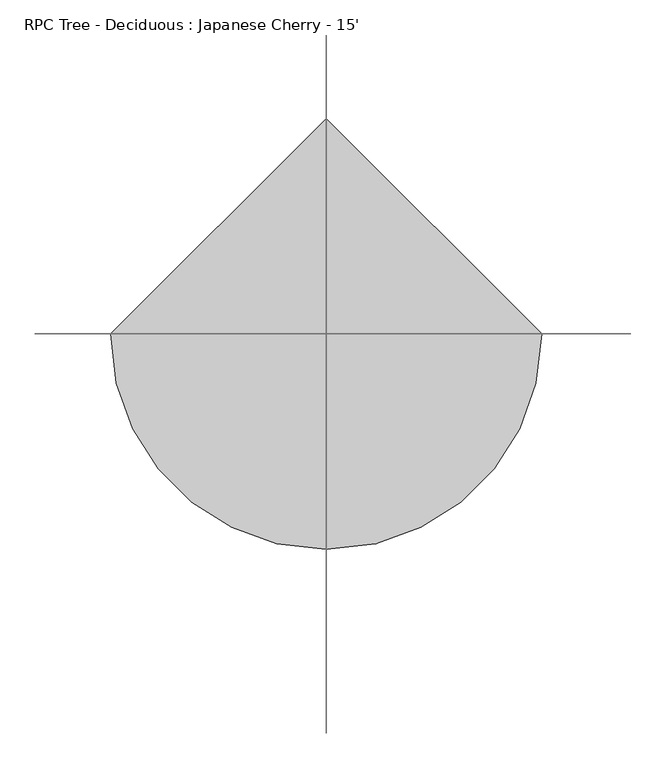
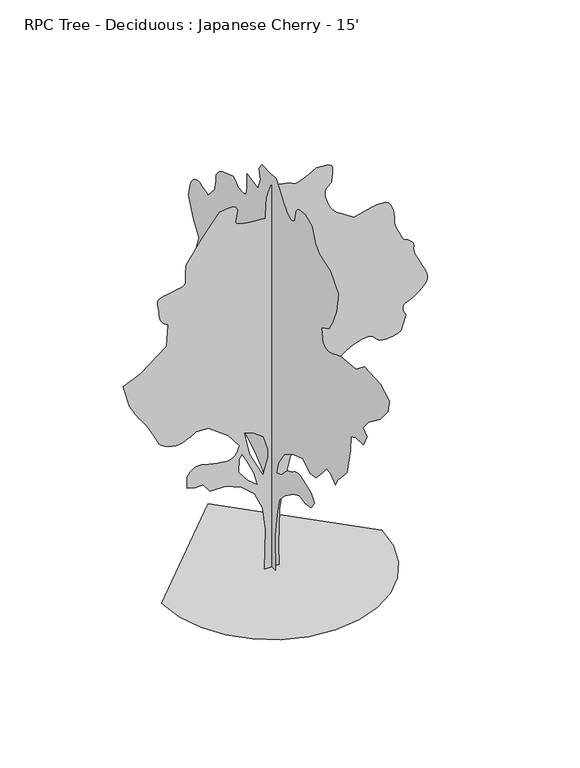
"""IFC4 building model written with IfcOpenShell, lengths in millimetres: geographic element geometry, RPC Tree - Deciduous : Japanese Cherry - 15'."""

from ifc_helpers import new_model, si_unit, origin, place, context, project, spatial, triangles, source, transform, mapped, element, save


def rpc_tree_deciduous_japanese_cherry_15_4daa029f(model_context):
    return source(origin(), model_context, "Body", "Tessellation", [
        triangles([(-0.0056056, 151.5314393, 0.0119075), (-0.0056056, -146.4956366, 0.0119075), (-0.0056056, -119.4024502, 799.2624058), (-0.0056056, -200.6820093, 1327.5829193), (-0.0056056, -295.5089247, 1733.9832584), (-0.0056056, -512.2574678, 1964.2750156), (-0.0056056, -837.3726522, 2194.5718597), (-0.0056056, -1054.1211954, 2289.3952869), (-0.0056056, -1270.8696659, 2248.7551804), (-0.0056056, -1501.1615685, 2289.3952869), (-0.0056056, -1623.0815975, 2465.5038689), (-0.0056056, -1501.1615685, 2628.0640045), (-0.0056056, -1067.669569, 2777.0755486), (-0.0056056, -1029.9911276, 2774.0379433), (-0.0056056, -992.6683331, 2770.1669586), (-0.0056056, -956.0567596, 2764.6347382), (-0.0056056, -920.5119816, 2756.618367), (-0.0056056, -886.3895731, 2745.2850471), (-0.0056056, -854.0400942, 2729.8011086), (-0.0056056, -823.8293655, 2709.343927), (-0.0056056, -793.6134773, 2687.3069), (-0.0056056, -761.2690853, 2667.3982315), (-0.0056056, -727.1466768, 2649.2728844), (-0.0056056, -691.6018988, 2632.5648926), (-0.0056056, -654.9903254, 2616.9286377), (-0.0056056, -617.6675308, 2601.9984444), (-0.0056056, -579.9891621, 2587.4237526), (-0.0056056, -376.7884838, 2370.6753548), (-0.0056056, -173.5888229, 2289.3952869), (-0.0056056, -254.8688908, 2573.8754517), (-0.0056056, -485.161738, 2912.5440239), (-0.0056056, -810.2809919, 3115.7444115), (-0.0056056, -1189.5895981, 3237.6642952), (-0.0056056, -1460.5214619, 3061.5558586), (-0.0056056, -1677.270005, 3088.6527512), (-0.0056056, -1907.5619076, 3332.4878677), (-0.0056056, -2083.6703442, 3549.2362656), (-0.0056056, -2246.2253929, 3535.6879646), (-0.0056056, -2422.3338295, 3373.1327705), (-0.0056056, -2530.705703, 3562.7845665), (-0.0056056, -2652.6255867, 3698.2481003), (-0.0056056, -2869.3742752, 3928.544799), (-0.0056056, -3004.8375183, 4538.1453804), (-0.0056056, -3018.3861099, 4863.2656517), (-0.0056056, -3208.0428474, 4944.5406326), (-0.0056056, -3506.0665169, 4971.6372345), (-0.0056056, -3627.9864006, 5229.0005951), (-0.0056056, -3478.9748566, 5350.9204788), (-0.0056056, -3682.1749535, 5594.7608276), (-0.0056056, -4142.7584679, 5947.0085129), (-0.0056056, -4440.7870789, 6299.2050385), (-0.0056056, -4494.9703995, 6583.6853485), (-0.0056056, -4156.3070595, 6773.3220291), (-0.0056056, -3533.1581772, 6800.4488617), (-0.0056056, -3221.5862068, 6556.6090942), (-0.0056056, -2625.5339264, 6488.8417191), (-0.0056056, -2544.569101, 6457.0913315), (-0.0056056, -2465.5038689, 6426.4083206), (-0.0056056, -2390.2231441, 6397.8589005), (-0.0056056, -2320.6372753, 6372.509285), (-0.0056056, -2258.6307404, 6351.4274323), (-0.0056056, -2206.1035686, 6335.6795563), (-0.0056056, -2164.9453251, 6326.2812927), (-0.0056056, -2128.100045, 6325.7731842), (-0.0056056, -2089.1160873, 6333.8000198), (-0.0056056, -2050.8485104, 6347.2619888), (-0.0056056, -2016.1317341, 6363.1116028), (-0.0056056, -1987.8157299, 6378.2496323), (-0.0056056, -1968.7402954, 6389.5785919), (-0.0056056, -1961.7452282, 6394.0486679), (-0.0056056, -1894.0134613, 6719.1689392), (-0.0056056, -2178.4937714, 6868.1656586), (-0.0056056, -2313.9621014, 7084.9291718), (-0.0056056, -2462.9737907, 7437.1256973), (-0.0056056, -2544.2540039, 7884.1664337), (-0.0056056, -2232.6820335, 8236.3629593), (-0.0056056, -1826.2818398, 8385.410257), (-0.0056056, -1663.7217041, 8534.4069763), (-0.0056056, -1541.8015297, 8859.5272476), (-0.0056056, -1257.321365, 8967.8834244), (-0.0056056, -1210.9917074, 8967.6805298), (-0.0056056, -1165.3783579, 8966.3085205), (-0.0056056, -1121.182291, 8962.5494476), (-0.0056056, -1079.1198875, 8955.2853561), (-0.0056056, -1039.9022232, 8943.1948151), (-0.0056056, -1004.2405918, 8925.2621887), (-0.0056056, -972.8411276, 8900.1672089), (-0.0056056, -947.3648483, 8868.7726135), (-0.0056056, -928.2894865, 8833.1108368), (-0.0056056, -914.5480288, 8793.8934631), (-0.0056056, -905.0687382, 8751.8309143), (-0.0056056, -898.7899063, 8707.6347748), (-0.0056056, -894.6395056, 8662.016629), (-0.0056056, -891.5610598, 8615.6868988), (-0.0056056, -868.1828356, 8589.8803345), (-0.0056056, -843.8496552, 8566.1062042), (-0.0056056, -817.6266191, 8546.3957794), (-0.0056056, -788.558844, 8532.6797562), (-0.0056056, -755.7014019, 8527.0405655), (-0.0056056, -718.0991913, 8531.4606445), (-0.0056056, -674.8125166, 8547.9706833), (-0.0056056, -631.9220387, 8571.9482895), (-0.0056056, -595.4323691, 8597.3990616), (-0.0056056, -564.2716258, 8624.018367), (-0.0056056, -537.372977, 8651.6027298), (-0.0056056, -513.6747869, 8679.8475174), (-0.0056056, -492.1126945, 8708.6004135), (-0.0056056, -471.6148905, 8737.6067825), (-0.0056056, -281.9620771, 8995.0108383), (-0.0056056, -160.0419754, 9144.0075577), (-0.0056056, 43.1582941, 9130.4438507), (-0.0056056, 368.2779568, 9144.0075577), (-0.0056056, 490.1975498, 8981.4471313), (-0.0056056, 436.0111771, 8751.1704895), (-0.0056056, 530.8400908, 8493.7670151), (-0.0056056, 950.783753, 8575.0469376), (-0.0056056, 950.783753, 8277.0029205), (-0.0056056, 953.9028214, 8230.8766663), (-0.0056056, 958.3275513, 8186.3247345), (-0.0056056, 965.3582268, 8145.1260864), (-0.0056056, 976.3005821, 8108.9562012), (-0.0056056, 992.4498871, 8079.3399857), (-0.0056056, 1015.121977, 8058.054657), (-0.0056056, 1045.6121218, 8046.7262787), (-0.0056056, 1080.4457514, 8042.510257), (-0.0056056, 1115.2793083, 8041.1382477), (-0.0056056, 1150.1129379, 8042.1038864), (-0.0056056, 1184.9464949, 8044.9990585), (-0.0056056, 1219.7800518, 8049.3173996), (-0.0056056, 1254.6187683, 8054.5496384), (-0.0056056, 1289.4523979, 8060.2899857), (-0.0056056, 1321.4004478, 8091.8874756), (-0.0056056, 1353.4705833, 8121.7583267), (-0.0056056, 1385.7793671, 8148.0724182), (-0.0056056, 1418.4387108, 8169.0531143), (-0.0056056, 1451.5756416, 8182.9214539), (-0.0056056, 1485.3068676, 8187.8996384), (-0.0056056, 1519.7441551, 8182.2098694), (-0.0056056, 1885.504533, 8060.2899857), (-0.0056056, 1937.4018013, 8025.3397934), (-0.0056056, 1987.1654789, 7989.6780167), (-0.0056056, 2032.6619751, 7952.5942337), (-0.0056056, 2071.7627861, 7913.3762787), (-0.0056056, 2102.3292343, 7871.3137299), (-0.0056056, 2122.2326706, 7825.6955841), (-0.0056056, 2129.3445911, 7775.8096756), (-0.0056056, 2130.9245819, 7724.7052368), (-0.0056056, 2135.3491665, 7675.7843857), (-0.0056056, 2142.1411938, 7628.6419144), (-0.0056056, 2150.8280182, 7582.9220306), (-0.0056056, 2160.9371395, 7538.2177826), (-0.0056056, 2171.9963482, 7494.2762787), (-0.0056056, 2183.5280571, 7450.6894043), (-0.0056056, 2440.9164162, 7166.2090942), (-0.0056056, 2519.1941963, 7200.4994431), (-0.0056056, 2596.8827682, 7231.7411407), (-0.0056056, 2673.3827499, 7256.836702), (-0.0056056, 2748.1043518, 7272.6863159), (-0.0056056, 2820.458947, 7276.1913345), (-0.0056056, 2889.8518044, 7264.3042694), (-0.0056056, 2955.6884834, 7233.9258911), (-0.0056056, 3012.8387741, 7186.9863144), (-0.0056056, 3057.9034653, 7128.6172028), (-0.0056056, 3092.8943527, 7060.7992493), (-0.0056056, 3119.8287552, 6985.4119904), (-0.0056056, 3140.722538, 6904.3349625), (-0.0056056, 3157.588369, 6819.4482834), (-0.0056056, 3172.4371719, 6732.6820679), (-0.0056056, 2996.3287354, 6272.1287842), (-0.0056056, 2779.5852791, 5974.0847672), (-0.0056056, 2955.6884834, 5486.4046509), (-0.0056056, 2793.1283478, 5229.0005951), (-0.0056056, 2726.7786186, 5205.6328354), (-0.0056056, 2662.917691, 5181.299437), (-0.0056056, 2604.0302971, 5155.0865021), (-0.0056056, 2552.605529, 5126.0289734), (-0.0056056, 2511.1374207, 5093.1612122), (-0.0056056, 2482.1104134, 5055.5640884), (-0.0056056, 2468.0080765, 5012.2771957), (-0.0056056, 2463.3906258, 4966.2270996), (-0.0056056, 2460.9012428, 4920.8833557), (-0.0056056, 2460.189949, 4876.1384125), (-0.0056056, 2460.9012428, 4831.8661148), (-0.0056056, 2462.679332, 4787.9443771), (-0.0056056, 2465.1684242, 4744.2665199), (-0.0056056, 2468.0080765, 4700.7005745), (-0.0056056, 2413.8249012, 4483.9571182), (-0.0056056, 2034.5162224, 4524.5970795), (-0.0056056, 2002.9998322, 4461.0105537), (-0.0056056, 1973.9726795, 4399.0803223), (-0.0056056, 1949.9189152, 4340.4722717), (-0.0056056, 1933.3327183, 4286.8377548), (-0.0056056, 1926.6982395, 4239.8423676), (-0.0056056, 1932.5047165, 4201.1328117), (-0.0056056, 1953.2361546, 4172.3851479), (-0.0056056, 1986.8454403, 4148.5293365), (-0.0056056, 2028.0392921, 4124.2011703), (-0.0056056, 2074.4450352, 4100.5842979), (-0.0056056, 2123.6956627, 4078.862368), (-0.0056056, 2173.4187904, 4060.2187386), (-0.0056056, 2221.2469757, 4045.8422905), (-0.0056056, 2264.8079796, 4036.9166725), (-0.0056056, 2304.2644375, 4029.134008), (-0.0056056, 2341.5873047, 4017.8006882), (-0.0056056, 2377.1320827, 4003.5053398), (-0.0056056, 2411.2544186, 3986.8380432), (-0.0056056, 2444.3150459, 3968.3923668), (-0.0056056, 2476.6595833, 3948.7633324), (-0.0056056, 2508.6483284, 3928.544799), (-0.0056056, 2820.2252403, 4091.1049347), (-0.0056056, 2909.7959358, 4113.9701088), (-0.0056056, 2996.8824806, 4134.7066338), (-0.0056056, 3078.9905502, 4151.1759773), (-0.0056056, 3153.635994, 4161.2445488), (-0.0056056, 3218.3300102, 4162.7839897), (-0.0056056, 3270.5829254, 4153.6653603), (-0.0056056, 3307.900415, 4131.7451866), (-0.0056056, 3332.589315, 4099.949453), (-0.0056056, 3349.4499138, 4063.1801857), (-0.0056056, 3359.7978287, 4022.2658226), (-0.0056056, 3364.9338524, 3978.0292786), (-0.0056056, 3366.1579056, 3931.3085838), (-0.0056056, 3364.7763039, 3882.9263626), (-0.0056056, 3362.0889679, 3833.7165756), (-0.0056056, 3315.525531, 3784.7808998), (-0.0056056, 3268.251091, 3738.3395485), (-0.0056056, 3219.5540634, 3696.8662079), (-0.0056056, 3168.7237358, 3662.8607254), (-0.0056056, 3115.048233, 3638.8119026), (-0.0056056, 3057.8220749, 3627.1992393), (-0.0056056, 2996.3287354, 3630.5164787), (-0.0056056, 2931.2030594, 3644.8115364), (-0.0056056, 2865.1274414, 3661.9564201), (-0.0056056, 2800.4741203, 3678.1464203), (-0.0056056, 2739.6156258, 3689.6018257), (-0.0056056, 2684.9143135, 3692.5228683), (-0.0056056, 2638.7470734, 3683.1248955), (-0.0056056, 2603.4765518, 3657.608139), (-0.0056056, 2576.8168419, 3624.7505516), (-0.0056056, 2554.4240227, 3595.4439102), (-0.0056056, 2535.5824402, 3569.1042389), (-0.0056056, 2519.5906837, 3545.1315742), (-0.0056056, 2505.7272858, 3522.9320572), (-0.0056056, 2493.2861847, 3501.9211304), (-0.0056056, 2481.5566681, 3481.504644), (-0.0056056, 2527.7236176, 3475.3832153), (-0.0056056, 2572.2345634, 3467.3668442), (-0.0056056, 2613.42827, 3455.5559372), (-0.0056056, 2649.643792, 3438.0604935), (-0.0056056, 2679.2245445, 3412.9803383), (-0.0056056, 2700.5148148, 3378.4211105), (-0.0056056, 2711.8484253, 3332.4878677), (-0.0056056, 2716.4711082, 3278.6600487), (-0.0056056, 2718.9604912, 3221.9824036), (-0.0056056, 2719.6714943, 3162.9374611), (-0.0056056, 2718.9604912, 3101.9978668), (-0.0056056, 2717.182402, 3039.635685), (-0.0056056, 2714.6933098, 2976.3287933), (-0.0056056, 2711.8484253, 2912.5440239), (-0.0056056, 2642.2625565, 2860.6873055), (-0.0056056, 2573.144101, 2811.198175), (-0.0056056, 2504.9752968, 2766.4532318), (-0.0056056, 2438.2292255, 2728.8157036), (-0.0056056, 2373.3830383, 2700.6572479), (-0.0056056, 2310.8989162, 2684.3451622), (-0.0056056, 2251.2647655, 2682.2522667), (-0.0056056, 2191.625528, 2689.6335022), (-0.0056056, 2129.1464928, 2699.8645638), (-0.0056056, 2064.2952187, 2712.4632133), (-0.0056056, 1997.5490021, 2726.9562241), (-0.0056056, 1929.3804886, 2742.8770546), (-0.0056056, 1860.2669746, 2759.7376534), (-0.0056056, 1790.6760189, 2777.0755486), (-0.0056056, 1384.2756798, 2682.2522667), (-0.0056056, 910.1437191, 2438.4122086), (-0.0056056, 639.2118553, 2289.3952869), (-0.0056056, 327.6379229, 2032.0117241), (-0.0056056, 137.9845917, 1639.1598312), (-0.0056056, 83.798219, 1083.7426432), (-0.0056056, 137.9845917, 528.3305783), (160.4204407, 0.0005103, 0.0), (-164.6993219, 0.0005103, 0.0), (-137.6061356, 0.0004465, 921.1724064), (-205.3388472, 0.000404, 1449.4927746), (-381.4458303, 0.0003827, 1828.7963665), (-665.9275938, 0.0003827, 2086.1850163), (-1018.1395254, 0.0003615, 2235.1967056), (-1356.8030834, 0.0003615, 2235.1967056), (-1519.368306, 0.0003615, 2438.3968025), (-1695.4716557, 0.0003615, 2438.3968025), (-1871.5802376, 0.0003615, 2479.0367638), (-1871.5802376, 0.0003402, 2736.4254135), (-1836.5078144, 0.0003402, 2782.4351051), (-1800.0130943, 0.0003402, 2825.8385605), (-1760.6785767, 0.000319, 2864.0301247), (-1717.0768776, 0.000319, 2894.4035614), (-1667.7857002, 0.000319, 2914.3474022), (-1611.3873985, 0.000319, 2921.261515), (-1546.4599663, 0.000319, 2912.5338501), (-1469.3658348, 0.000319, 2893.021669), (-1380.897543, 0.000319, 2870.9032516), (-1286.2671272, 0.0003402, 2848.5514183), (-1190.6920017, 0.0003402, 2828.3279434), (-1099.378898, 0.0003402, 2812.6102982), (-1017.5451576, 0.0003402, 2803.7608383), (-950.4027443, 0.0003402, 2804.1570351), (-897.088048, 0.0003402, 2816.2830391), (-852.3027729, 0.0003402, 2839.7833488), (-814.6244041, 0.000319, 2872.7627312), (-782.6304995, 0.000319, 2913.321302), (-754.9089357, 0.000319, 2959.5696419), (-730.0270969, 0.000319, 3009.6078667), (-706.5676277, 0.000319, 3061.5456848), (-950.4027443, 0.0002977, 3386.6659561), (-1397.4430447, 0.0002764, 3711.7862274), (-1668.3799953, 0.0002764, 3725.3295868), (-1712.0985477, 0.0002764, 3699.2640266), (-1756.8838955, 0.0002764, 3673.5542587), (-1803.8077755, 0.0002764, 3648.5554939), (-1853.9220131, 0.0002764, 3624.6185829), (-1908.3086643, 0.0002764, 3602.1089104), (-1968.0240601, 0.0002764, 3581.3723854), (-2034.1403732, 0.0002977, 3562.7694511), (-2110.2031723, 0.0002977, 3556.3329254), (-2194.8004795, 0.0002977, 3569.3277718), (-2281.5313774, 0.0002764, 3597.9585823), (-2364.0001808, 0.0002764, 3638.4412857), (-2435.8010307, 0.0002764, 3686.9804741), (-2490.5380966, 0.0002764, 3739.7871346), (-2521.8155479, 0.0002764, 3793.0664406), (-2549.1103935, 0.0002764, 3859.4923279), (-2592.5141396, 0.0002552, 3947.9607651), (-2646.5806068, 0.0002552, 4048.9918076), (-2705.8641975, 0.0002552, 4153.0964996), (-2764.90914, 0.0002552, 4250.8050705), (-2818.2643135, 0.0002339, 4332.6390289), (-2860.4841202, 0.0002339, 4389.1184303), (-2896.110434, 0.0002339, 4434.1017311), (-2933.1538124, 0.0002339, 4486.9083916), (-2971.3857811, 0.0002339, 4546.2277359), (-3010.5627502, 0.0002339, 4610.7589714), (-3050.4510132, 0.0002126, 4679.207119), (-3090.8165726, 0.0002126, 4750.2559799), (-3131.4161293, 0.0002126, 4822.6102844), (-3280.4329056, 0.0001914, 5337.4079315), (-2887.5757805, 0.0001701, 5499.9677765), (-2318.6205379, 0.0001488, 5947.0085129), (-2291.5237907, 0.0001063, 6434.6380508), (-2331.8894955, 0.0001063, 6463.9496338), (-2370.5941097, 0.0001063, 6494.6326447), (-2405.9813393, 0.0001063, 6528.1608307), (-2436.390239, 0.0001063, 6565.9561981), (-2460.1646599, 0.0001063, 6609.4407532), (-2475.6485985, 0.0001063, 6660.0376648), (-2481.1805283, 0.0001063, 6719.1183609), (-2486.0779037, 8.51e-05, 6785.6660431), (-2497.1318802, 8.51e-05, 6855.0589005), (-2508.9023827, 8.51e-05, 6923.5372787), (-2515.9330582, 8.51e-05, 6987.2409485), (-2512.7730766, 8.51e-05, 7042.4096741), (-2493.9721893, 8.51e-05, 7085.2338043), (-2454.0839264, 8.51e-05, 7112.005426), (-2384.2185688, 8.51e-05, 7128.8206787), (-2288.2877964, 6.38e-05, 7145.4318741), (-2180.0329216, 6.38e-05, 7163.1616058), (-2073.200489, 6.38e-05, 7183.5830338), (-1981.5318111, 6.38e-05, 7207.9670105), (-1918.7734325, 6.38e-05, 7237.8372803), (-1898.6718979, 6.38e-05, 7274.5658524), (-1902.8983841, 6.38e-05, 7318.7619919), (-1904.2801311, 6.38e-05, 7369.3589035), (-1903.2894939, 6.38e-05, 7425.2897919), (-1900.4091465, 6.38e-05, 7485.436702), (-1896.1065022, 4.25e-05, 7548.8351578), (-1890.8537704, 4.25e-05, 7614.3672043), (-1885.1234516, 4.25e-05, 7680.9660461), (-1546.4599663, 2.13e-05, 8168.6467438), (-1153.6079281, -2.13e-05, 8656.32686), (-1069.9961712, -2.13e-05, 8670.2463593), (-989.8235212, -2.13e-05, 8680.7619965), (-916.5191294, -2.13e-05, 8684.4193314), (-853.5270441, -2.13e-05, 8677.7139267), (-804.2764166, -2.13e-05, 8657.2919174), (-772.2063538, -2.13e-05, 8619.7000259), (-760.7509483, 0.0, 8561.4832306), (-766.3998768, 0.0, 8495.9006058), (-779.3945778, 0.0, 8438.090181), (-793.8115757, 0.0, 8387.6961639), (-803.7226713, 0.0, 8344.1098709), (-803.2096212, 0.0, 8306.92435), (-786.3440083, 0.0, 8275.6820709), (-747.2076616, 0.0, 8249.9266663), (-687.8477674, 0.0, 8229.0477081), (-615.6863291, 0.0, 8212.4870911), (-532.8670383, 2.13e-05, 8199.4314926), (-441.5173817, 2.13e-05, 8189.2710663), (-343.7679339, 2.13e-05, 8181.1942337), (-241.7533214, 2.13e-05, 8174.5394073), (-137.6061356, 2.13e-05, 8168.6467438), (-124.0587793, 0.0, 8534.4069763), (-120.8990158, -2.13e-05, 8586.2735779), (-112.0521903, -2.13e-05, 8637.378598), (-98.4662281, -2.13e-05, 8687.92435), (-81.0885461, -2.13e-05, 8738.0131531), (-60.8670833, -2.13e-05, 8787.7467453), (-38.7503736, -2.13e-05, 8837.2257019), (-15.6855285, -2.13e-05, 8886.6035019), (76.7715585, -2.13e-05, 8869.1284058), (166.622097, -2.13e-05, 8851.4498337), (251.2590275, -2.13e-05, 8833.3143127), (328.0763045, -2.13e-05, 8814.416629), (394.4668742, -2.13e-05, 8794.6044662), (447.8241915, -2.13e-05, 8773.5731918), (485.5411843, -2.13e-05, 8751.1199112), (534.634881, -2.13e-05, 8744.5668228), (614.5281149, -2.13e-05, 8765.038829), (711.2513535, -2.13e-05, 8803.0376724), (810.8194765, -2.13e-05, 8849.1133484), (899.2470732, -2.13e-05, 8893.7152771), (962.5541101, -4.25e-05, 8927.4469391), (986.765423, -4.25e-05, 8940.8071701), (1006.2776768, -4.25e-05, 8941.2135406), (1056.5950996, -4.25e-05, 8940.6548538), (1125.3935892, -4.25e-05, 8936.5399887), (1200.35413, -4.25e-05, 8926.2784058), (1269.1526196, -2.13e-05, 8907.2284058), (1319.4700424, -2.13e-05, 8876.7988678), (1338.9823689, -2.13e-05, 8832.3998337), (1338.1899754, -2.13e-05, 8780.9396027), (1335.9800812, -2.13e-05, 8730.9013779), (1332.5815968, -2.13e-05, 8682.0822647), (1328.2381119, -2.13e-05, 8634.178212), (1323.1836239, -2.13e-05, 8586.984581), (1317.6514034, 0.0, 8540.2490616), (1311.8856216, 0.0, 8493.7670151), (1277.3670891, 0.0, 8467.3506042), (1244.7482952, 0.0, 8439.4616089), (1215.9142267, 0.0, 8408.4228058), (1192.7697092, 0.0, 8372.8121887), (1177.2096851, 0.0, 8331.0542725), (1171.128879, 0.0, 8281.5753159), (1176.4222332, 0.0, 8222.7992523), (1191.1898638, 2.13e-05, 8157.6735764), (1211.6470453, 2.13e-05, 8091.3287888), (1236.8489227, 2.13e-05, 8025.8984802), (1265.8353802, 2.13e-05, 7963.5668198), (1297.6667221, 2.13e-05, 7906.4673981), (1331.3979481, 2.13e-05, 7856.6832275), (1366.0740292, 4.25e-05, 7816.3990585), (1406.8309891, 4.25e-05, 7779.6199081), (1458.2557571, 4.25e-05, 7739.2340012), (1518.5605064, 4.25e-05, 7695.901181), (1585.9824085, 4.25e-05, 7650.2318756), (1658.7279682, 4.25e-05, 7602.7341934), (1735.0297062, 4.25e-05, 7554.1185562), (1813.1144749, 4.25e-05, 7504.8424942), (1948.9740601, 4.25e-05, 7542.0280151), (2081.3995525, 4.25e-05, 7575.7590958), (2206.951918, 4.25e-05, 7602.5818771), (2322.2020054, 4.25e-05, 7619.1424942), (2423.7004612, 4.25e-05, 7621.9365097), (2508.0233665, 4.25e-05, 7607.5600616), (2571.7267456, 4.25e-05, 7572.5587097), (2617.6192932, 4.25e-05, 7515.662764), (2651.8991776, 6.38e-05, 7442.4090958), (2676.2273438, 6.38e-05, 7359.6560074), (2692.2650276, 6.38e-05, 7274.3117981), (2701.6630005, 6.38e-05, 7193.2347702), (2706.0877304, 8.51e-05, 7123.283226), (2707.1952209, 8.51e-05, 7071.3654648), (2717.7006844, 8.51e-05, 7015.9938446), (2744.7923447, 8.51e-05, 6938.5741516), (2781.8357231, 8.51e-05, 6850.2836105), (2822.2012825, 0.0001063, 6762.1965454), (2859.2498932, 0.0001063, 6685.4884369), (2886.3415535, 0.0001063, 6631.2847687), (2896.8470169, 0.0001063, 6610.7616028), (2911.0252213, 0.0001063, 6605.1229935), (2947.2404526, 0.0001063, 6588.8158493), (2996.0188705, 0.0001063, 6562.8063904), (3047.8752983, 0.0001063, 6528.0085144), (3093.3312447, 0.0001063, 6485.3872787), (3122.9122879, 0.0001063, 6435.9077408), (3127.1387741, 0.0001276, 6380.4849609), (3121.8454926, 0.0001276, 6323.7924911), (3127.9311676, 0.0001276, 6268.7760818), (3143.4912643, 0.0001276, 6213.7590912), (3166.6357819, 0.0001276, 6157.1171997), (3195.4648361, 0.0001276, 6097.1226059), (3228.0887169, 0.0001488, 6032.1492462), (3262.6072495, 0.0001488, 5960.5210602), (3302.0228668, 0.0001488, 5882.8478943), (3345.7059563, 0.0001488, 5801.8220261), (3386.3052223, 0.0001488, 5719.1700943), (3416.4754738, 0.0001701, 5636.5187439), (3428.8808212, 0.0001701, 5555.4922943), (3416.1603767, 0.0001701, 5477.8191284), (3370.9788322, 0.0001701, 5405.124147), (3310.1206284, 0.0001914, 5341.7768509), (3253.9967285, 0.0001914, 5289.8085114), (3200.7174225, 0.0001914, 5247.2884323), (3148.3883492, 0.0001914, 5212.3888184), (3095.1093338, 0.0001914, 5183.1789734), (3038.9903755, 0.0001914, 5157.7282013), (2978.1269394, 0.0001914, 5134.2075439), (2926.5091599, 0.0001914, 5107.0295517), (2896.923175, 0.0001914, 5072.7293198), (2885.7064178, 0.0001914, 5032.5265411), (2889.1861473, 0.0002126, 4987.5787033), (2903.6794487, 0.0002126, 4939.0799194), (2925.5185226, 0.0002126, 4888.2138382), (2951.0352791, 0.0002126, 4836.158876), (2842.6584641, 0.0002339, 4497.4900131), (2804.5482903, 0.0002339, 4480.2335083), (2764.1827309, 0.0002339, 4463.9214226), (2719.3159927, 0.0002339, 4449.50457), (2667.6982132, 0.0002339, 4437.9323112), (2607.0734253, 0.0002339, 4430.1545883), (2535.191185, 0.0002339, 4427.1117508), (2449.8065712, 0.0002339, 4429.7583916), (2373.1086365, 0.0002339, 4447.3302841), (2320.5814648, 0.0002339, 4482.4432571), (2279.9008083, 0.0002339, 4526.0853607), (2238.7476517, 0.0002339, 4569.2501678), (2184.7980377, 0.0002339, 4602.940844), (2105.7277187, 0.0002339, 4618.1454391), (1989.2178246, 0.0002339, 4605.8618866), (1854.5062798, 0.0002339, 4567.5941643), (1730.9250149, 0.0002339, 4513.6852455), (1621.3290882, 0.0002339, 4448.3970795), (1528.5529198, 0.0002339, 4376.0070213), (1455.4517132, 0.0002339, 4300.7671371), (1404.8548016, 0.0002552, 4226.9544914), (1379.6224754, 0.0002552, 4158.8266731), (1379.0687302, 0.0002552, 4098.1204948), (1398.4184212, 0.0002552, 4043.1040855), (1434.359396, 0.0002552, 3992.8272125), (1483.5694736, 0.0002552, 3946.345166), (1542.7311241, 0.0002764, 3902.7030624), (1608.5324856, 0.0002764, 3860.9556107), (1677.6459995, 0.0002764, 3820.1581009), (1717.9710091, 0.0002764, 3793.8536018), (1756.4012215, 0.0002764, 3766.4825981), (1791.0367527, 0.0002764, 3736.9829453), (1819.9876019, 0.0002764, 3704.283197), (1841.3541756, 0.0002764, 3667.3159767), (1853.241386, 0.0002764, 3625.0147797), (1853.7544361, 0.0002764, 3576.3177521), (1848.3443012, 0.0002977, 3516.9580032), (1843.6451694, 0.0002977, 3444.8016518), (1839.5355366, 0.0002977, 3361.9822884), (1835.9033455, 0.0002977, 3270.6285622), (1832.6215691, 0.000319, 3172.8790054), (1829.5838184, 0.000319, 3070.8674995), (1826.6576889, 0.000319, 2966.7171707), (1756.9142715, 0.000319, 2915.058696), (1686.6934124, 0.000319, 2866.9561089), (1615.5226112, 0.0003402, 2825.9606461), (1542.9293678, 0.0003402, 2795.6279045), (1468.4462688, 0.0003402, 2779.5140625), (1391.585844, 0.0003402, 2781.1700661), (1311.8856216, 0.0003402, 2804.1570351), (1231.7942894, 0.0003402, 2834.6473251), (1153.831461, 0.0003402, 2857.3194878), (1077.6415621, 0.000319, 2873.4737343), (1002.8791924, 0.000319, 2884.4111481), (929.1835453, 0.000319, 2891.4418236), (856.1991194, 0.000319, 2895.8665535), (783.5652534, 0.000319, 2898.9855492), (553.2733872, 0.0003402, 2749.9737144), (404.2611528, 0.0003615, 2411.3051422), (255.2473379, 0.0003827, 1842.3448128), (173.9677787, 0.0004253, 1286.9326389), (146.8740927, 0.0004678, 474.1330507), (-191.7925083, 0.0001701, 2194.5567444), (-83.4192541, 0.0001488, 2573.8652779), (-83.4192541, 0.0001276, 2763.5170738), (-178.2451521, 0.0001063, 3088.6373451), (-422.0848469, 0.0001063, 3264.7457817), (-611.7391863, 0.0001063, 3332.4776939), (-489.8190845, 0.0001276, 2790.6139664), (-313.7115927, 0.0001276, 2018.4532494), (-394.9916605, 0.0001276, 2316.4767735), (-544.0074921, 0.0001063, 2641.5968994), (-652.3792202, 8.51e-05, 2844.797287), (-720.1109144, 8.51e-05, 2749.9737144), (-733.659288, 0.0001063, 2451.9451035), (-530.4591185, 0.0001276, 2194.5567444), (-2425.8340519, 0.0, 0.0091858), (-2361.7041, -555.8388193, 0.0091858), (-2179.0575451, -1066.2928362, 0.0091858), (-1892.5250347, -1516.7266068, 0.0091858), (-1516.7266068, -1892.5250347, 0.0091858), (-1066.2928362, -2179.0575451, 0.0091858), (-555.8388193, -2361.7041, 0.0091858), (0.000106, -2425.8340519, 0.0091858), (555.8388193, -2361.7041, 0.0091858), (1066.2928362, -2179.0575451, 0.0091858), (1516.7266068, -1892.5250347, 0.0091858), (1892.5250347, -1516.7266068, 0.0091858), (2179.0575451, -1066.2928362, 0.0091858), (2361.7041, -555.8388193, 0.0091858), (2425.8340519, 0.0002126, 0.0091858), (-0.0003181, 2425.8340519, 0.0091858)], [[38, 39, 40], [115, 116, 117], [1, 2, 3], [280, 1, 3], [279, 280, 3], [279, 3, 4], [278, 279, 4], [278, 4, 5], [186, 187, 188], [277, 278, 5], [46, 47, 48], [45, 46, 48], [277, 5, 6], [185, 186, 188], [10, 11, 12], [9, 10, 12], [9, 12, 13], [8, 9, 13], [8, 13, 14], [8, 14, 15], [8, 15, 16], [8, 16, 17], [8, 17, 18], [8, 18, 19], [8, 19, 20], [8, 20, 21], [7, 8, 21], [7, 21, 22], [7, 22, 23], [7, 23, 24], [7, 24, 25], [7, 25, 26], [6, 7, 26], [6, 26, 27], [6, 27, 28], [277, 6, 28], [277, 28, 29], [51, 52, 53], [50, 51, 53], [50, 53, 54], [50, 54, 55], [49, 50, 55], [49, 55, 56], [48, 49, 56], [48, 56, 57], [45, 48, 57], [44, 45, 57], [44, 57, 58], [44, 58, 59], [44, 59, 60], [44, 60, 61], [44, 61, 62], [44, 62, 63], [276, 277, 29], [276, 29, 30], [184, 185, 188], [183, 184, 188], [44, 63, 64], [115, 117, 118], [111, 112, 113], [111, 113, 114], [182, 183, 188], [109, 110, 111], [109, 111, 114], [108, 109, 114], [108, 114, 115], [107, 108, 115], [106, 107, 115], [105, 106, 115], [104, 105, 115], [115, 118, 119], [170, 171, 172], [170, 172, 173], [170, 173, 174], [170, 174, 175], [74, 75, 76], [74, 76, 77], [73, 74, 77], [72, 73, 77], [71, 72, 77], [258, 259, 260], [181, 182, 188], [78, 79, 80], [170, 175, 176], [103, 104, 115], [78, 80, 81], [44, 64, 65], [275, 276, 30], [275, 30, 31], [274, 275, 31], [78, 81, 82], [78, 82, 83], [78, 83, 84], [78, 84, 85], [78, 85, 86], [78, 86, 87], [78, 87, 88], [78, 88, 89], [78, 89, 90], [78, 90, 91], [78, 91, 92], [78, 92, 93], [78, 93, 94], [78, 94, 95], [78, 95, 96], [71, 77, 78], [71, 78, 96], [71, 96, 97], [71, 97, 98], [71, 98, 99], [71, 99, 100], [115, 119, 120], [180, 181, 188], [38, 40, 41], [223, 224, 225], [33, 34, 35], [33, 35, 36], [33, 36, 37], [102, 103, 115], [179, 180, 188], [44, 65, 66], [170, 176, 177], [71, 100, 101], [43, 44, 66], [42, 43, 66], [41, 42, 66], [38, 41, 66], [37, 38, 66], [33, 37, 66], [33, 66, 67], [33, 67, 68], [33, 68, 69], [33, 69, 70], [32, 33, 70], [31, 32, 70], [274, 31, 70], [273, 274, 70], [273, 70, 71], [273, 71, 101], [273, 101, 102], [273, 102, 115], [273, 115, 120], [273, 120, 121], [273, 121, 122], [273, 122, 123], [273, 123, 124], [273, 124, 125], [273, 125, 126], [273, 126, 127], [273, 127, 128], [273, 128, 129], [273, 129, 130], [273, 130, 131], [272, 273, 131], [271, 272, 131], [270, 271, 131], [269, 270, 131], [268, 269, 131], [268, 131, 132], [268, 132, 133], [268, 133, 134], [167, 168, 169], [257, 258, 260], [257, 260, 261], [256, 257, 261], [256, 261, 262], [255, 256, 262], [255, 262, 263], [254, 255, 263], [254, 263, 264], [254, 264, 265], [254, 265, 266], [254, 266, 267], [254, 267, 268], [253, 254, 268], [252, 253, 268], [251, 252, 268], [250, 251, 268], [249, 250, 268], [248, 249, 268], [247, 248, 268], [246, 247, 268], [245, 246, 268], [166, 167, 169], [165, 166, 169], [164, 165, 169], [163, 164, 169], [162, 163, 169], [161, 162, 169], [160, 161, 169], [159, 160, 169], [158, 159, 169], [157, 158, 169], [156, 157, 169], [155, 156, 169], [154, 155, 169], [154, 169, 170], [154, 170, 177], [153, 154, 177], [153, 177, 178], [153, 178, 179], [153, 179, 188], [222, 223, 225], [222, 225, 226], [221, 222, 226], [220, 221, 226], [219, 220, 226], [218, 219, 226], [217, 218, 226], [216, 217, 226], [215, 216, 226], [214, 215, 226], [213, 214, 226], [212, 213, 226], [212, 226, 227], [212, 227, 228], [212, 228, 229], [212, 229, 230], [212, 230, 231], [211, 212, 231], [211, 231, 232], [211, 232, 233], [210, 211, 233], [209, 210, 233], [209, 233, 234], [209, 234, 235], [209, 235, 236], [209, 236, 237], [209, 237, 238], [209, 238, 239], [209, 239, 240], [208, 209, 240], [208, 240, 241], [207, 208, 241], [206, 207, 241], [206, 241, 242], [205, 206, 242], [204, 205, 242], [204, 242, 243], [203, 204, 243], [202, 203, 243], [202, 243, 244], [201, 202, 244], [201, 244, 245], [201, 245, 268], [200, 201, 268], [199, 200, 268], [198, 199, 268], [197, 198, 268], [196, 197, 268], [195, 196, 268], [194, 195, 268], [153, 188, 189], [153, 189, 190], [152, 153, 190], [152, 190, 191], [151, 152, 191], [136, 137, 138], [135, 136, 138], [135, 138, 139], [134, 135, 139], [134, 139, 140], [134, 140, 141], [134, 141, 142], [134, 142, 143], [134, 143, 144], [134, 144, 145], [134, 145, 146], [134, 146, 147], [134, 147, 148], [134, 148, 149], [134, 149, 150], [134, 150, 151], [134, 151, 191], [134, 191, 192], [134, 192, 193], [268, 134, 193], [194, 268, 193], [583, 580, 581], [574, 281, 575], [580, 583, 584], [573, 574, 575], [583, 581, 575], [580, 584, 585], [572, 573, 575], [582, 583, 575], [582, 575, 281], [571, 572, 575], [571, 575, 576], [281, 282, 283], [570, 571, 576], [570, 576, 577], [344, 345, 346], [290, 291, 292], [406, 407, 408], [570, 577, 578], [290, 292, 293], [289, 290, 293], [289, 293, 294], [289, 294, 295], [289, 295, 296], [289, 296, 297], [289, 297, 298], [289, 298, 299], [289, 299, 300], [289, 300, 301], [289, 301, 302], [289, 302, 303], [288, 289, 303], [287, 288, 303], [287, 303, 304], [287, 304, 305], [287, 305, 306], [286, 287, 306], [286, 306, 307], [286, 307, 308], [286, 308, 309], [569, 570, 578], [554, 555, 556], [405, 406, 408], [343, 344, 346], [512, 513, 514], [511, 512, 514], [511, 514, 515], [511, 515, 516], [511, 516, 517], [510, 511, 517], [510, 517, 518], [510, 518, 519], [510, 519, 520], [510, 520, 521], [510, 521, 522], [510, 522, 523], [510, 523, 524], [509, 510, 524], [509, 524, 525], [508, 509, 525], [434, 435, 436], [342, 343, 346], [507, 508, 525], [507, 525, 526], [405, 408, 409], [404, 405, 409], [403, 404, 409], [403, 409, 410], [402, 403, 410], [401, 402, 410], [400, 401, 410], [400, 410, 411], [399, 400, 411], [399, 411, 412], [399, 412, 413], [399, 413, 414], [399, 414, 415], [377, 378, 379], [341, 342, 346], [341, 346, 347], [340, 341, 347], [339, 340, 347], [338, 339, 347], [337, 338, 347], [336, 337, 347], [335, 336, 347], [334, 335, 347], [333, 334, 347], [377, 379, 380], [377, 380, 381], [377, 381, 382], [377, 382, 383], [377, 383, 384], [377, 384, 385], [377, 385, 386], [377, 386, 387], [377, 387, 388], [377, 388, 389], [377, 389, 390], [377, 390, 391], [376, 377, 391], [376, 391, 392], [375, 376, 392], [374, 375, 392], [373, 374, 392], [372, 373, 392], [372, 392, 393], [371, 372, 393], [370, 371, 393], [369, 370, 393], [369, 393, 394], [369, 394, 395], [369, 395, 396], [332, 333, 347], [369, 396, 397], [426, 427, 428], [426, 428, 429], [425, 426, 429], [425, 429, 430], [424, 425, 430], [424, 430, 431], [423, 424, 431], [423, 431, 432], [422, 423, 432], [422, 432, 433], [421, 422, 433], [420, 421, 433], [419, 420, 433], [418, 419, 433], [418, 433, 434], [418, 434, 436], [418, 436, 437], [418, 437, 438], [418, 438, 439], [417, 418, 439], [417, 439, 440], [416, 417, 440], [416, 440, 441], [415, 416, 441], [399, 415, 441], [399, 441, 442], [399, 442, 443], [399, 443, 444], [399, 444, 445], [399, 445, 446], [399, 446, 447], [399, 447, 448], [399, 448, 449], [369, 397, 398], [331, 332, 347], [368, 369, 398], [360, 361, 362], [359, 360, 362], [359, 362, 363], [358, 359, 363], [358, 363, 364], [357, 358, 364], [357, 364, 365], [356, 357, 365], [355, 356, 365], [355, 365, 366], [354, 355, 366], [353, 354, 366], [352, 353, 366], [351, 352, 366], [350, 351, 366], [349, 350, 366], [348, 349, 366], [348, 366, 367], [348, 367, 368], [348, 368, 398], [347, 348, 398], [347, 398, 399], [347, 399, 449], [347, 449, 450], [347, 450, 451], [347, 451, 452], [331, 347, 452], [331, 452, 453], [331, 453, 454], [331, 454, 455], [331, 455, 456], [330, 331, 456], [329, 330, 456], [328, 329, 456], [327, 328, 456], [326, 327, 456], [325, 326, 456], [324, 325, 456], [323, 324, 456], [322, 323, 456], [321, 322, 456], [320, 321, 456], [319, 320, 456], [318, 319, 456], [317, 318, 456], [316, 317, 456], [315, 316, 456], [314, 315, 456], [314, 456, 457], [314, 457, 458], [314, 458, 459], [314, 459, 460], [314, 460, 461], [314, 461, 462], [314, 462, 463], [314, 463, 464], [314, 464, 465], [314, 465, 466], [314, 466, 467], [314, 467, 468], [314, 468, 469], [314, 469, 470], [314, 470, 471], [314, 471, 472], [314, 472, 473], [314, 473, 474], [314, 474, 475], [314, 475, 476], [314, 476, 477], [314, 477, 478], [314, 478, 479], [314, 479, 480], [314, 480, 481], [314, 481, 482], [314, 482, 483], [314, 483, 484], [314, 484, 485], [314, 485, 486], [314, 486, 487], [314, 487, 488], [314, 488, 489], [314, 489, 490], [314, 490, 491], [314, 491, 492], [314, 492, 493], [314, 493, 494], [314, 494, 495], [314, 495, 496], [314, 496, 497], [314, 497, 498], [314, 498, 499], [314, 499, 500], [314, 500, 501], [314, 501, 502], [580, 585, 586], [554, 556, 557], [553, 554, 557], [553, 557, 558], [553, 558, 559], [553, 559, 560], [553, 560, 561], [553, 561, 562], [553, 562, 563], [552, 553, 563], [552, 563, 564], [551, 552, 564], [550, 551, 564], [550, 564, 565], [549, 550, 565], [549, 565, 566], [548, 549, 566], [547, 548, 566], [546, 547, 566], [545, 546, 566], [544, 545, 566], [543, 544, 566], [542, 543, 566], [541, 542, 566], [540, 541, 566], [539, 540, 566], [538, 539, 566], [538, 566, 567], [537, 538, 567], [537, 567, 568], [537, 568, 569], [537, 569, 578], [536, 537, 578], [535, 536, 578], [535, 578, 579], [534, 535, 579], [534, 579, 580], [533, 534, 580], [532, 533, 580], [507, 526, 527], [506, 507, 527], [531, 532, 580], [506, 527, 528], [530, 531, 580], [281, 283, 284], [582, 281, 284], [582, 284, 285], [582, 285, 286], [588, 582, 286], [587, 588, 286], [587, 286, 309], [586, 587, 309], [586, 309, 310], [586, 310, 311], [586, 311, 312], [586, 312, 313], [580, 586, 313], [580, 313, 314], [530, 580, 314], [529, 530, 314], [502, 503, 504], [502, 504, 505], [314, 502, 505], [529, 314, 505], [529, 505, 506], [529, 506, 528], [603, 604, 589], [602, 603, 589], [602, 589, 590], [601, 602, 590], [601, 590, 591], [601, 591, 592], [600, 601, 592], [599, 600, 592], [599, 592, 593], [599, 593, 594], [599, 594, 595], [599, 595, 596], [599, 596, 597], [599, 597, 598]], closed=False),
    ])


if __name__ == "__main__":
    model = new_model("IFC4")
    model_context = context("Model", 3, world=origin())
    ifc_project = project(units=[si_unit("LENGTHUNIT", "METRE", prefix="MILLI")], contexts=[model_context])
    site = spatial("IfcSite", under=ifc_project)
    building = spatial("IfcBuilding", under=site)
    placement = place(None, origin())
    rpc_tree_deciduous_japanese_cherry_15_shape = rpc_tree_deciduous_japanese_cherry_15_4daa029f(model_context)
    element("IfcGeographicElement", 1, ObjectType="RPC Tree - Deciduous : Japanese Cherry - 15'", at=placement, inside=building, context=model_context, shape_type="MappedRepresentation", body=[
        mapped(rpc_tree_deciduous_japanese_cherry_15_shape, transform((0.0, 0.0, 0.0), x_axis=(1.0, 0.0, 0.0), y_axis=(0.0, 1.0, 0.0), z_axis=(0.0, 0.0, 1.0))),
    ])
    save(model, "model.ifc")

# Revit data of these elements
# Type "RPC Tree - Deciduous : Japanese Cherry - 15'"
#   built-in parameter 1005198 = "{2, 15},{39, RPC-16-FXGW-2MQ0-PN7K-A000-ST1L-LVER-AU},{1, 0},{1, 0},{2, 35},{1, 8},{5, Color},{1, 0},{1, 0},{3, 0.8},{3, 0.8},{3, 0.8},{1, 8},{7, BBoxMin},{1, 0},{1, 0},{1, 0},{1, 0},{1, 0},{1, 8},{7, BBoxMax},{1, 0},{1, 0},{1, 0},{1, 0},{1, 0},{2, 11},{9, RPCTypeId},{1, 0},{1, 0},{39, RPC-16-FXGW-2MQ0-PN7K-A000-ST1L-LVER-AU},{1, 6},{14, RPCPlantHeight},{1, 0},{1, 0},{2, 15},{2, 11},{7, keyword},{1, 0},{1, 0},{207, :Geometry:RPC:Japanese Flowering Cherry:Prunus serrulata Lindl:A landscape tree:valued for its abundant showy flowers; native to China and Japan.  Hardy only in the mildest parts of Canada and farther south.},{2, 11},{8, category},{1, 0},{1, 0},{16, :Trees [General]},{2, 11},{12, LocalizedUID},{1, 0},{1, 0},{25, Japanese Flowering Cherry},{2, 14},{6, Height},{1, 0},{1, 0},{2, 15},{1, 2},{16, Cast Reflections},{1, 0},{1, 0},{1, 0},{1, 2},{12, Cast Shadows},{1, 0},{1, 0},{1, 1},{1, 2},{9, Lock View},{1, 0},{1, 0},{1, 0},{1, 4},{5, ViewC},{1, 0},{1, 0},{1, 0},{2, 11},{20, AdvancedUIDefinition},{1, 0},{1, 0},{0, },{2, 11},{10, AssetLibID},{1, 0},{1, 0},{36, 4D3F6E72-3F99-4203-98E9-AF80B3C7A7A4},{2, 11},{10, BaseSchema},{1, 0},{1, 0},{9, RPCSchema},{2, 11},{12, ExchangeGUID},{1, 0},{1, 0},{0, },{1, 2},{6, Hidden},{1, 0},{1, 0},{1, 0},{1, 4},{11, RPCCategory},{1, 0},{1, 0},{1, 0},{2, 11},{8, RPCImage},{1, 0},{1, 0},{0, },{1, 4},{13, SchemaVersion},{1, 0},{1, 0},{1, 4},{2, 11},{12, UIDefinition},{1, 0},{1, 0},{0, },{2, 11},{6, UIName},{1, 0},{1, 0},{39, RPC-16-FXGW-2MQ0-PN7K-A000-ST1L-LVER-AU},{2, 11},{11, VersionGUID},{1, 0},{1, 0},{9, RPCSchema},{2, 11},{9, assettype},{1, 0},{1, 0},{11, RPCGeometry},{2, 11},{11, description},{1, 0},{1, 0},{0, },{2, 11},{9, localname},{1, 0},{1, 0},{3, RPC},{2, 11},{9, localtype},{1, 0},{1, 0},{3, RPC},{1, 4},{8, revision},{1, 0},{1, 0},{1, 1},{2, 11},{9, thumbnail},{1, 0},{1, 0},{0, },{1, 4},{7, version},{1, 0},{1, 0},{1, 1},{1, 2},{20, RPC_Cast Reflections},{1, 0},{1, 0},{1, 1},{1, 2},{16, RPC_Cast Shadows},{1, 0},{1, 0},{1, 1},{1, 2},{13, RPC_Lock View},{1, 0},{1, 0},{1, 0},{1, 4},{9, RPC_ViewC},{1, 0},{1, 0},{1, 0},{21, assetlibrary_base.fbx},{1, 5},"
#   built-in parameter 1005195 = "RPC-16-FXGW-2MQ0-PN7K-A000-ST1L-LVER-AU"
#   Type Comments = "Japanese Cherry"
#   Assembly Code = "G2050500"
#   Height = 30' - 0"
#   Default Elevation = 0
